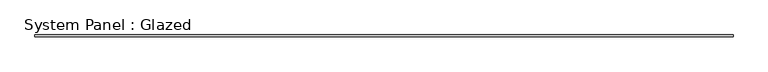
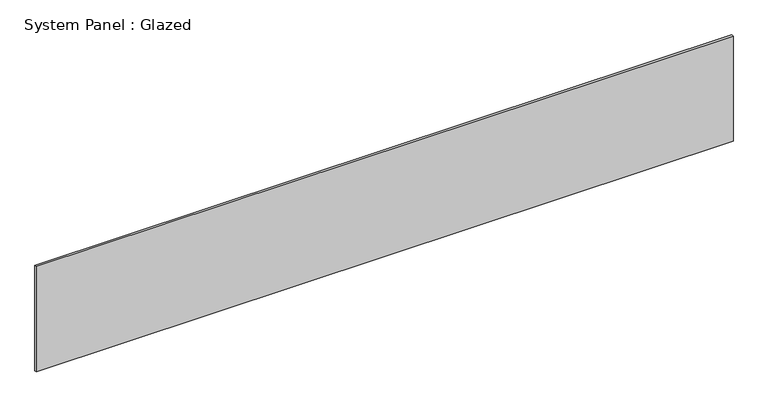
"""IFC4 building model written with IfcOpenShell, lengths in millimetres: plate geometry, System Panel : Glazed."""

from ifc_helpers import new_model, si_unit, origin, origin_with_axes, place, context, project, spatial, polyline, outline, extrude, source, transform, mapped, element, save


def system_panel_glazed_1f6fd899(model_context):
    return source(origin(), model_context, "Body", "SweptSolid", [
        extrude(outline(polyline([(4568.825, 19.05), (-4568.825, 19.05), (-4568.825, 44.45), (4568.825, 44.45), (4568.825, 19.05)])), origin_with_axes(), (0.0, 0.0, 1.0), 1460.5),
    ])


if __name__ == "__main__":
    model = new_model("IFC4")
    model_context = context("Model", 3, world=origin())
    ifc_project = project(units=[si_unit("LENGTHUNIT", "METRE", prefix="MILLI")], contexts=[model_context])
    site = spatial("IfcSite", under=ifc_project)
    building = spatial("IfcBuilding", under=site)
    placement = place(None, origin())
    system_panel_glazed_shape = system_panel_glazed_1f6fd899(model_context)
    element("IfcPlate", 1, ObjectType="System Panel : Glazed", at=placement, inside=building, context=model_context, shape_type="MappedRepresentation", body=[
        mapped(system_panel_glazed_shape, transform((0.0, 0.0, 0.0), x_axis=(1.0, 0.0, 0.0), y_axis=(0.0, 1.0, 0.0), z_axis=(0.0, 0.0, 1.0))),
    ])
    save(model, "model.ifc")

# Revit data of these elements
# Type "System Panel : Glazed"
#   Construction Type Id = "GSP4R"
#   Analytic Construction = "1/8 in Pilkington single glazing"
#   Visual Light Transmittance = 0.9
#   Solar Heat Gain Coefficient = 0.86
#   Heat Transfer Coefficient (U) = 1.18115 BTU/(h·ft²·°F)
# Element 1 (IfcPlate, "System Panel : Glazed")
#   Materials on its faces: "Glass"
# Materials
#   "Glass": class "Glass", colour RGB 0 128 192, transparency 0.75, Description = "Soda Lime Glass", Cost = 0
